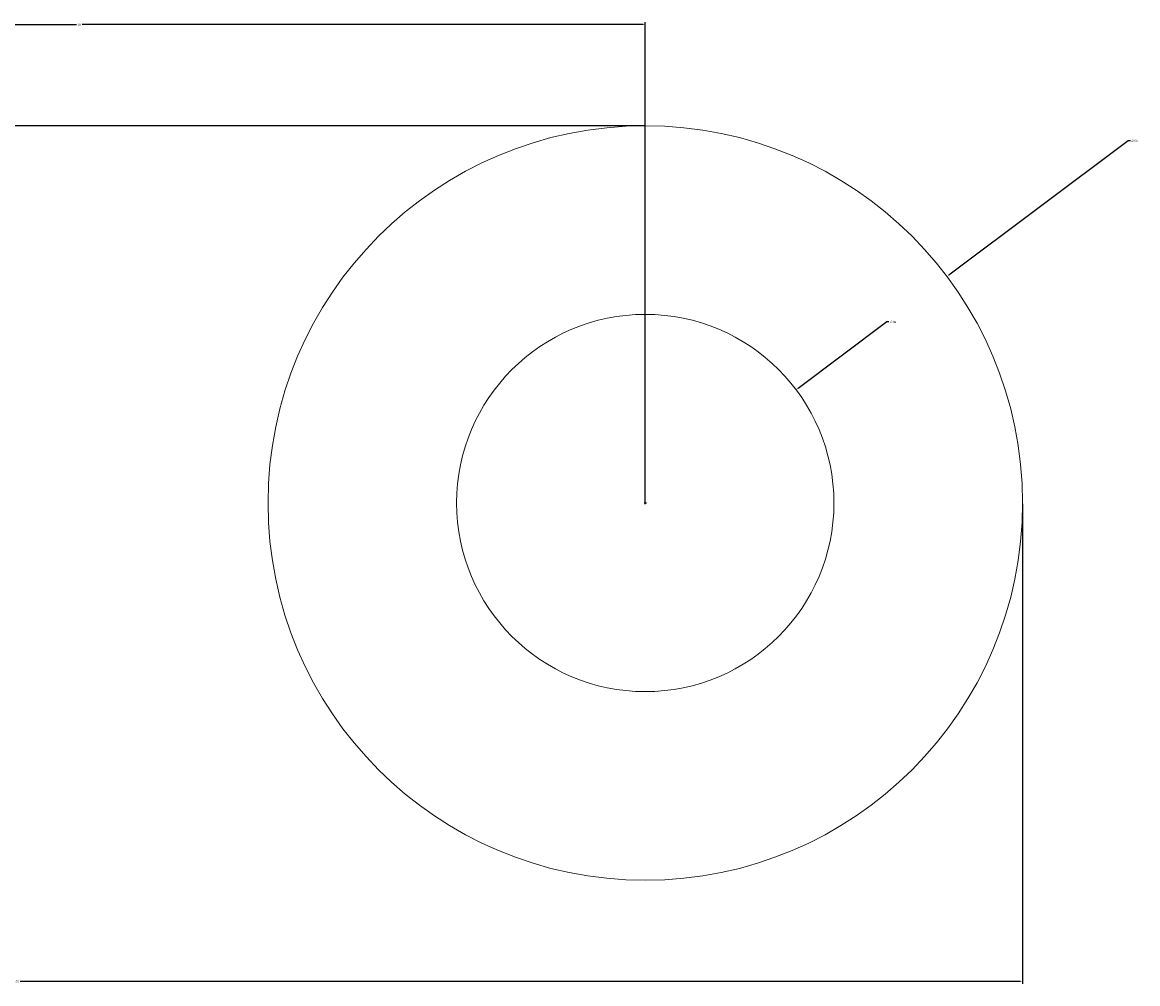
# Model space of a CAD drawing. Units: millimetres. Extents: x -48 to 129, y -118 to -41.
# Tile 6 of 6: x 40 to 129, y -118 to -41. Entities that reach past the tile are written whole.
import ezdxf

# ---------------------------------------------------------------- set-up
doc = ezdxf.new("R2010")
doc.units = ezdxf.units.MM
doc.layers.add('M-CONS', color=8, linetype='Continuous', lineweight=18)
doc.layers.add('M-DIMS', color=2, linetype='Continuous', lineweight=18)
doc.styles.get("Standard").update_dxf_attribs({"font": 'arial.ttf'})
doc.dimstyles.get("Standard").update_dxf_attribs({"dimtxt": 0.18, "dimasz": 0.18, "dimexe": 0.18, "dimexo": 0.0625, "dimgap": 0.09, "dimtad": 0, "dimtih": 1, "dimtoh": 1, "dimdec": 4, "dimzin": 0, "dimdsep": 46, "dimtxsty": 'Standard', "dimcen": 0.09, "dimadec": 0, "dimazin": 0, "dimtfac": 1, "dimtdec": 4, "dimtofl": 0, "dimtmove": 0, "dimatfit": 3, "dimfxl": 1, "dimtolj": 1, "dimtzin": 0, "dimarcsym": 0})

# ---------------------------------------------------------------- blocks, each defined once
blk = doc.blocks.new('*D1')
at = {"layer": 'Defpoints', "color": 0, "transparency": 16777216}
for p in [(120, -79.442), (-40, -99.442), (120, -117.492)]:
    blk.add_point(p, dxfattribs=at)
at = {"layer": 'M-DIMS', "color": 0, "lineweight": -2, "transparency": 16777216}
for p, q in [((120, -79.505), (120, -117.672)), ((-40, -99.505), (-40, -117.672)), ((-39.82, -117.492), (39.72, -117.492)), ((119.82, -117.492), (40.28, -117.492))]:
    blk.add_line(p, q, dxfattribs=at)
at = {"layer": 'M-DIMS', "color": 0, "transparency": 16777216}
for points in [[(-39.82, -117.462), (-39.82, -117.522), (-40, -117.492)], [(119.82, -117.462), (119.82, -117.522), (120, -117.492)]]:
    blk.add_solid(points, dxfattribs=at)
at = {"layer": 'M-DIMS', "color": 0, "transparency": 16777216, "insert": (40, -117.492), "char_height": 0.18, "attachment_point": 5}
blk.add_mtext('\\A1;160', dxfattribs=at)
blk = doc.blocks.new('*D3')
at = {"layer": 'Defpoints', "color": 0, "transparency": 16777216}
for p in [(90, -41.392), (0, -59.442), (90, -79.442)]:
    blk.add_point(p, dxfattribs=at)
at = {"layer": 'M-DIMS', "color": 0, "lineweight": -2, "transparency": 16777216}
for p, q in [((0, -59.38), (0, -41.212)), ((0.18, -41.392), (44.781, -41.392)), ((89.82, -41.392), (45.219, -41.392)), ((90, -79.38), (90, -41.212))]:
    blk.add_line(p, q, dxfattribs=at)
at = {"layer": 'M-DIMS', "color": 0, "transparency": 16777216}
for points in [[(0.18, -41.362), (0.18, -41.422), (0, -41.392)], [(89.82, -41.362), (89.82, -41.422), (90, -41.392)]]:
    blk.add_solid(points, dxfattribs=at)
at = {"layer": 'M-DIMS', "color": 0, "transparency": 16777216, "insert": (45, -41.392), "char_height": 0.18, "attachment_point": 5}
blk.add_mtext('\\A1;90', dxfattribs=at)
blk = doc.blocks.new('*D8')
at = {"layer": 'Defpoints', "color": 0, "transparency": 16777216}
for p in [(-48.05, -49.442), (90, -49.442), (0, -59.442)]:
    blk.add_point(p, dxfattribs=at)
at = {"layer": 'M-DIMS', "color": 0, "lineweight": -2, "transparency": 16777216}
for p, q in [((89.938, -49.442), (-48.23, -49.442)), ((-48.05, -49.622), (-48.05, -54.26)), ((-48.05, -59.262), (-48.05, -54.624)), ((-0.062, -59.442), (-48.23, -59.442))]:
    blk.add_line(p, q, dxfattribs=at)
at = {"layer": 'M-DIMS', "color": 0, "transparency": 16777216}
for points in [[(-48.08, -49.622), (-48.02, -49.622), (-48.05, -49.442)], [(-48.08, -59.262), (-48.02, -59.262), (-48.05, -59.442)]]:
    blk.add_solid(points, dxfattribs=at)
at = {"layer": 'M-DIMS', "color": 0, "transparency": 16777216, "insert": (-48.05, -54.442), "char_height": 0.18, "attachment_point": 5}
blk.add_mtext('\\A1;10', dxfattribs=at)
blk = doc.blocks.new('*D10')
at = {"layer": 'Defpoints', "color": 0, "transparency": 16777216}
for p in [(102, -70.442), (78, -88.442)]:
    blk.add_point(p, dxfattribs=at)
at = {"layer": 'M-DIMS', "color": 0, "lineweight": -2, "transparency": 16777216}
for p, q in [((109.2, -65.042), (102.144, -70.334)), ((109.38, -65.042), (109.2, -65.042)), ((89.91, -79.442), (90.09, -79.442)), ((90, -79.532), (90, -79.352))]:
    blk.add_line(p, q, dxfattribs=at)
at = {"layer": 'M-DIMS', "color": 0, "transparency": 16777216}
blk.add_solid([(102.126, -70.31), (102.162, -70.358), (102, -70.442)], dxfattribs=at)
at = {"layer": 'M-DIMS', "color": 0, "transparency": 16777216, "insert": (109.696, -65.042), "char_height": 0.18, "attachment_point": 5}
blk.add_mtext('\\A1;∅30', dxfattribs=at)
blk = doc.blocks.new('*D11')
at = {"layer": 'Defpoints', "color": 0, "transparency": 16777216}
for p in [(114, -61.442), (66, -97.442)]:
    blk.add_point(p, dxfattribs=at)
at = {"layer": 'M-DIMS', "color": 0, "lineweight": -2, "transparency": 16777216}
for p, q in [((128.4, -50.642), (114.144, -61.334)), ((128.58, -50.642), (128.4, -50.642)), ((89.91, -79.442), (90.09, -79.442)), ((90, -79.532), (90, -79.352))]:
    blk.add_line(p, q, dxfattribs=at)
at = {"layer": 'M-DIMS', "color": 0, "transparency": 16777216}
blk.add_solid([(114.126, -61.31), (114.162, -61.358), (114, -61.442)], dxfattribs=at)
at = {"layer": 'M-DIMS', "color": 0, "transparency": 16777216, "insert": (128.896, -50.642), "char_height": 0.18, "attachment_point": 5}
blk.add_mtext('\\A1;∅60', dxfattribs=at)

msp = doc.modelspace()

# ---------------------------------------------------------------- linework, layer by layer
at = {"layer": 'M-CONS'}
for radius in [30, 15]:
    msp.add_circle((90, -79.442, 46.324), radius, dxfattribs=at)

# ---------------------------------------------------------------- dimensions: what is measured, and where the dimension line sits
at = {"layer": 'M-DIMS'}
for base, p1, p2, picture, middle in [((90, -41.392), (0, -59.442), (90, -79.442), '*D3', (45, -41.392)), ((120, -117.492), (-40, -99.442), (120, -79.442), '*D1', (40, -117.492))]:
    dim = msp.add_linear_dim(base=base, p1=p1, p2=p2, dimstyle='Standard', override={"dimdec": 0, "dimlfac": 1, "dimrnd": 0, "dimzin": 0, "dimdsep": 46, "dimlunit": 2}, dxfattribs=at)
    dim.commit()
    dim.dimension.update_dxf_attribs({"geometry": picture, "text_midpoint": middle})
dim = msp.add_linear_dim(base=(-48.05, -49.442), p1=(0, -59.442), p2=(90, -49.442), angle=90, dimstyle='Standard', override={"dimdec": 0, "dimlfac": 1, "dimrnd": 0, "dimzin": 0, "dimdsep": 46, "dimlunit": 2}, dxfattribs=at)
dim.commit()
dim.dimension.update_dxf_attribs({"geometry": '*D8', "text_midpoint": (-48.05, -54.442)})
for p1, p2, picture, middle in [((66, -97.442), (114, -61.442), '*D11', (128.896, -50.642)), ((78, -88.442), (102, -70.442), '*D10', (109.696, -65.042))]:
    dim = msp.add_diameter_dim_2p(p1=p1, p2=p2, dimstyle='Standard', override={"dimdec": 0, "dimlfac": 1, "dimrnd": 0, "dimzin": 0, "dimdsep": 46, "dimlunit": 2}, dxfattribs=at)
    dim.commit()
    dim.dimension.update_dxf_attribs({"geometry": picture, "text_midpoint": middle, "dimtype": 163})

doc.saveas('drawing.dxf')
